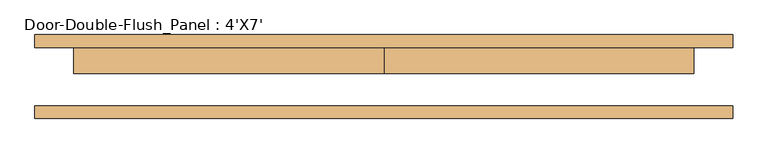
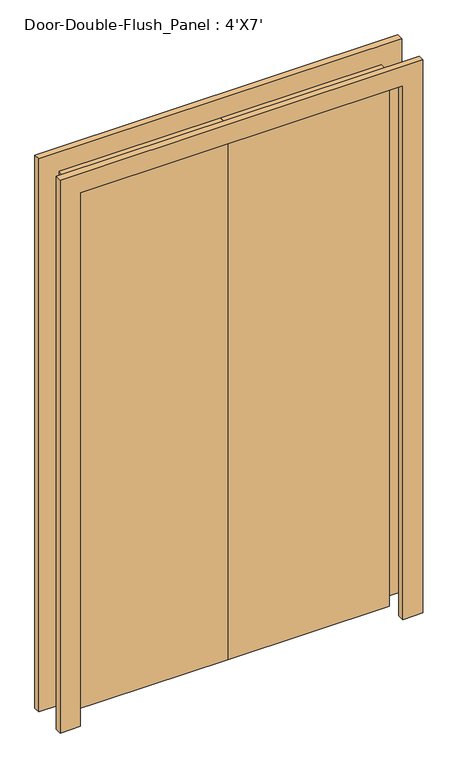
"""IFC4 building model written with IfcOpenShell, lengths in millimetres: door geometry, Door-Double-Flush_Panel : 4'X7'."""

from ifc_helpers import new_model, si_unit, frame, origin, origin_with_axes, place, context, project, spatial, polyline, outline, extrude, source, transform, mapped, element, save


def door_double_flush_panel_4_x7_eb8a45e1(model_context):
    return source(origin(), model_context, "Body", "SweptSolid", [
        extrude(outline(polyline([(2133.6, -609.6), (2133.6, 609.6), (0.0, 609.6), (0.0, 685.8), (2209.8, 685.8), (2209.8, -685.8), (0.0, -685.8), (0.0, -609.6), (2133.6, -609.6)])), frame((0.0, 57.15, 0.0), z_axis=(0.0, 1.0, 0.0), x_axis=(0.0, 0.0, 1.0)), (0.0, 0.0, 1.0), 25.4),
        extrude(outline(polyline([(2133.6, -609.6), (2133.6, 609.6), (0.0, 609.6), (0.0, 685.8), (2209.8, 685.8), (2209.8, -685.8), (0.0, -685.8), (0.0, -609.6), (2133.6, -609.6)])), frame((0.0, -82.55, 0.0), z_axis=(0.0, 1.0, 0.0), x_axis=(0.0, 0.0, 1.0)), (0.0, 0.0, 1.0), 25.4),
        extrude(outline(polyline([(-609.6, 57.15), (0.0, 57.15), (0.0, 6.35), (-609.6, 6.35), (-609.6, 57.15)])), origin_with_axes(), (0.0, 0.0, 1.0), 2133.6),
        extrude(outline(polyline([(0.0, 57.15), (609.6, 57.15), (609.6, 6.35), (0.0, 6.35), (0.0, 57.15)])), origin_with_axes(), (0.0, 0.0, 1.0), 2133.6),
    ])


if __name__ == "__main__":
    model = new_model("IFC4")
    model_context = context("Model", 3, world=origin())
    ifc_project = project(units=[si_unit("LENGTHUNIT", "METRE", prefix="MILLI")], contexts=[model_context])
    site = spatial("IfcSite", under=ifc_project)
    building = spatial("IfcBuilding", under=site)
    placement = place(None, origin())
    door_double_flush_panel_4_x7_shape = door_double_flush_panel_4_x7_eb8a45e1(model_context)
    element("IfcDoor", 1, ObjectType="Door-Double-Flush_Panel : 4'X7'", at=placement, inside=building, context=model_context, shape_type="MappedRepresentation", body=[
        mapped(door_double_flush_panel_4_x7_shape, transform((0.0, 0.0, 0.0), x_axis=(1.0, 0.0, 0.0), y_axis=(0.0, 1.0, 0.0), z_axis=(0.0, 0.0, 1.0))),
    ])
    save(model, "model.ifc")

# Revit data of these elements
# Type "Door-Double-Flush_Panel : 4'X7'"
#   Type Mark = "11"
#   Construction Type Id = "DOOR"
#   Assembly Code = "C1020"
#   Analytic Construction = "Wooden"
#   Thickness = 0' - 2"
#   Thermal Resistance (R) = 2.5876 (h·ft²·°F)/BTU
#   Swing Angle [instance default] = 90.00°
#   Panel Width = 2' - 0"
#   Heat Transfer Coefficient (U) = 0.3865 BTU/(h·ft²·°F)
#   Height = 7' - 0"
#   Trim Projection Ext = 0' - 1"
#   Trim Projection Int = 0' - 1"
#   Trim Width = 0' - 3"
#   Width = 4' - 0"
#   Define Thermal Properties by = 1
#   Panel Material = Wood - Birch - Solid Stained Light Low Gloss
#   Trim Material = Paint - Sienna
#   Visual Light Transmittance = 0
#   Solar Heat Gain Coefficient = 0
#   Function = (empty or 0)
#   Wall Closure = (empty or 0)
# Element 1 (IfcDoor, "Door-Double-Flush_Panel : 4'X7'")
#   Materials on its faces: "Paint - Sienna", "Wood - Birch - Solid Stained Light Low Gloss"
# Materials
#   "Wood - Birch - Solid Stained Light Low Gloss": class "Wood", colour RGB 210 159 95, transparency 0, Cost = 0
#   "Paint - Sienna": colour RGB 118 70 51, transparency 0, Cost = 0
